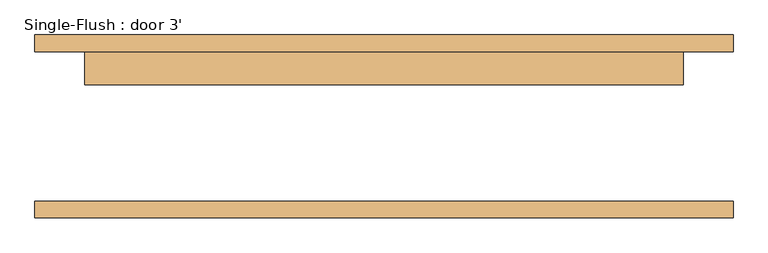
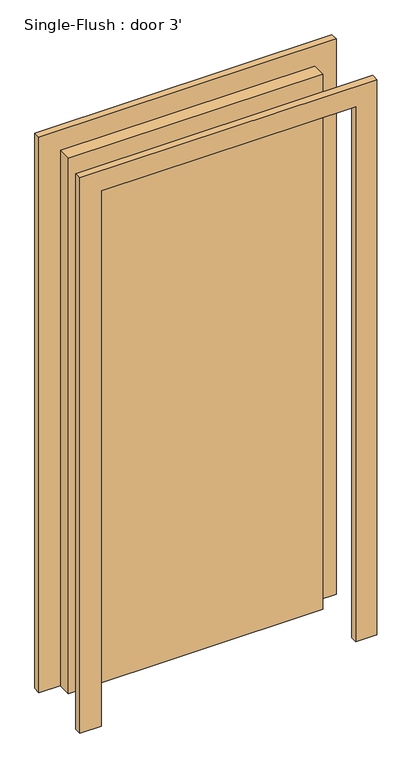
"""IFC4 building model written with IfcOpenShell, lengths in millimetres: door geometry, Single-Flush : door 3'."""

from ifc_helpers import new_model, si_unit, frame, origin, origin_with_axes, place, context, project, spatial, polyline, outline, extrude, source, transform, mapped, element, save


def single_flush_door_3_89fc3733(model_context):
    return source(origin(), model_context, "Body", "SweptSolid", [
        extrude(outline(polyline([(2108.2, -533.4), (0.0, -533.4), (0.0, -457.2), (2032.0, -457.2), (2032.0, 457.2), (0.0, 457.2), (0.0, 533.4), (2108.2, 533.4), (2108.2, -533.4)])), frame((0.0, 114.3, 0.0), z_axis=(0.0, 1.0, 0.0), x_axis=(0.0, 0.0, 1.0)), (0.0, 0.0, 1.0), 25.4),
        extrude(outline(polyline([(2108.2, 533.4), (2108.2, -533.4), (0.0, -533.4), (0.0, -457.2), (2032.0, -457.2), (2032.0, 457.2), (0.0, 457.2), (0.0, 533.4), (2108.2, 533.4)])), frame((0.0, -139.7, 0.0), z_axis=(0.0, 1.0, 0.0), x_axis=(0.0, 0.0, 1.0)), (0.0, 0.0, 1.0), 25.4),
        extrude(outline(polyline([(457.2, 63.5), (-457.2, 63.5), (-457.2, 114.3), (457.2, 114.3), (457.2, 63.5)])), origin_with_axes(), (0.0, 0.0, 1.0), 2032.0),
    ])


if __name__ == "__main__":
    model = new_model("IFC4")
    model_context = context("Model", 3, world=origin())
    ifc_project = project(units=[si_unit("LENGTHUNIT", "METRE", prefix="MILLI")], contexts=[model_context])
    site = spatial("IfcSite", under=ifc_project)
    building = spatial("IfcBuilding", under=site)
    placement = place(None, origin())
    single_flush_door_3_shape = single_flush_door_3_89fc3733(model_context)
    element("IfcDoor", 1, ObjectType="Single-Flush : door 3'", at=placement, inside=building, context=model_context, shape_type="MappedRepresentation", body=[
        mapped(single_flush_door_3_shape, transform((0.0, 0.0, 0.0), x_axis=(1.0, 0.0, 0.0), y_axis=(0.0, 1.0, 0.0), z_axis=(0.0, 0.0, 1.0))),
    ])
    save(model, "model.ifc")

# Revit data of these elements
# Type "Single-Flush : door 3'"
#   Type Mark = "9"
#   Construction Type Id = "MDOOR"
#   Assembly Code = "C1020"
#   Analytic Construction = "Metal"
#   Thickness = 0' - 2"
#   Heat Transfer Coefficient (U) = 0.651978 BTU/(h·ft²·°F)
#   Height = 6' - 8"
#   Trim Projection Ext = 0' - 1"
#   Trim Projection Int = 0' - 1"
#   Trim Width = 0' - 3"
#   Width = 3' - 0"
#   Define Thermal Properties by = 1
#   Door Material = Door - Panel
#   Frame Material = Door - Frame
#   Visual Light Transmittance = 0
#   Solar Heat Gain Coefficient = 0
#   Function = (empty or 0)
#   Wall Closure = (empty or 0)
# Element 1 (IfcDoor, "Single-Flush : door 3'")
#   Materials on its faces: "Door - Frame", "Door - Panel"
# Materials
#   "Door - Panel": class "Wood", colour RGB 210 159 95, transparency 0, Cost = 0
#   "Door - Frame": colour RGB 118 70 51, transparency 0, Cost = 0
